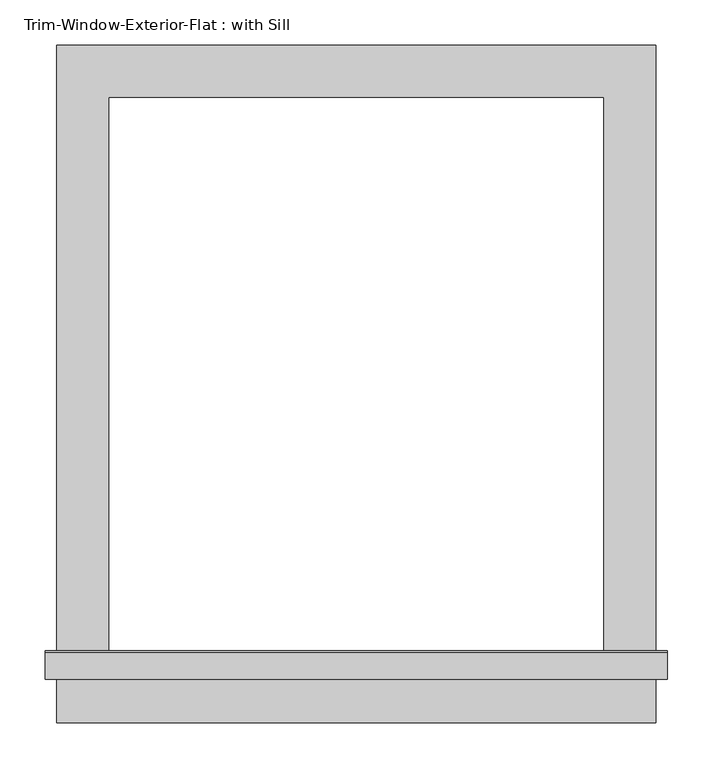
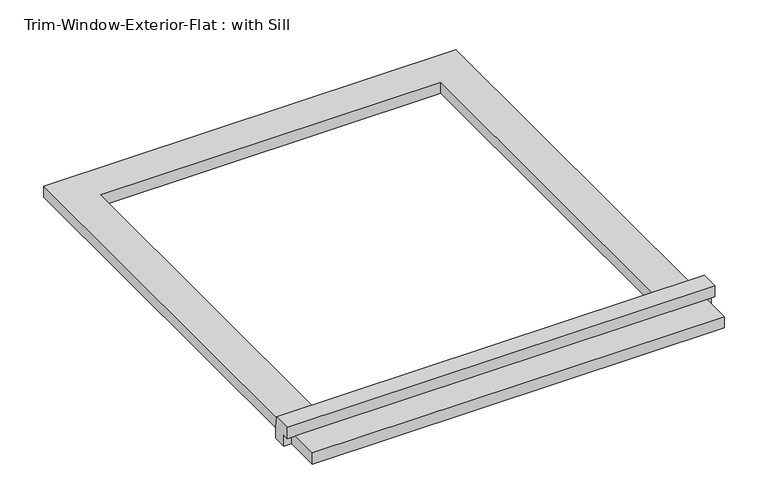
"""IFC4 building model written with IfcOpenShell, lengths in millimetres: proxy geometry, Trim-Window-Exterior-Flat : with Sill."""

from ifc_helpers import new_model, si_unit, frame, origin, origin_with_axes, place, context, project, spatial, polyline, outline, extrude, source, transform, mapped, element, save


def trim_window_exterior_flat_with_sill_575f95a5(model_context):
    return source(origin(), model_context, "Body", "SweptSolid", [
        extrude(outline(polyline([(330.2, -631.7823709), (330.2, -688.9323709), (-330.2, -688.9323709), (-330.2, -631.7823709), (330.2, -631.7823709)])), origin_with_axes(), (0.0, 0.0, 1.0), 19.05),
        extrude(outline(polyline([(-641.35, 38.1), (-612.0580645, 38.1), (-609.6, 19.05), (-609.6, 0.0), (-631.7823709, 0.0), (-631.7823709, 19.05), (-641.35, 19.05), (-641.35, 38.1)])), frame((-342.9, 0.0, 0.0), z_axis=(1.0, 0.0, 0.0), x_axis=(0.0, 1.0, 0.0)), (0.0, 0.0, 1.0), 685.8),
        extrude(outline(polyline([(-330.2, 57.15), (330.2, 57.15), (330.2, -609.6), (273.05, -609.6), (273.05, 0.0), (-273.05, 0.0), (-273.05, -609.6), (-330.2, -609.6), (-330.2, 57.15)])), origin_with_axes(), (0.0, 0.0, 1.0), 19.05),
    ])


if __name__ == "__main__":
    model = new_model("IFC4")
    model_context = context("Model", 3, world=origin())
    ifc_project = project(units=[si_unit("LENGTHUNIT", "METRE", prefix="MILLI")], contexts=[model_context])
    site = spatial("IfcSite", under=ifc_project)
    building = spatial("IfcBuilding", under=site)
    placement = place(None, origin())
    trim_window_exterior_flat_with_sill_shape = trim_window_exterior_flat_with_sill_575f95a5(model_context)
    element("IfcBuildingElementProxy", 1, Name="Trim-Window-Exterior-Flat : with Sill", ObjectType="Trim-Window-Exterior-Flat : with Sill", at=placement, inside=building, context=model_context, shape_type="MappedRepresentation", body=[
        mapped(trim_window_exterior_flat_with_sill_shape, transform((0.0, 0.0, 0.0), x_axis=(1.0, 0.0, 0.0), y_axis=(0.0, 1.0, 0.0), z_axis=(0.0, 0.0, 1.0))),
    ])
    save(model, "model.ifc")

# Revit data of these elements
# Type "Trim-Window-Exterior-Flat : with Sill"
#   Trim Width = 0' - 2 1/4"
#   Trim Thickness_Picture Frame = 0' - 1 1/4"
#   Trim Thickness_with Sill = 0' - 0 3/4"
#   Sill Thickness = 0' - 1 1/4"
#   Opening Width [instance default] = 2' - 0"
#   Opening Height [instance default] = 3' - 0"
#   Default Elevation = 4' - 0"
#   Sill = yes
#   Picture Frame = no
#   Trim Material [instance default] = none
# Element 1 (IfcBuildingElementProxy, "Trim-Window-Exterior-Flat : with Sill")
#   Opening Width = 1' - 9 1/2"
#   Opening Height = 2' - 0"
#   Trim Material = Clad - White
#   Materials on its faces: "Clad - White"
# Materials
#   "Clad - White": class "Wood", colour RGB 242 242 238, transparency 0, Cost = 0
